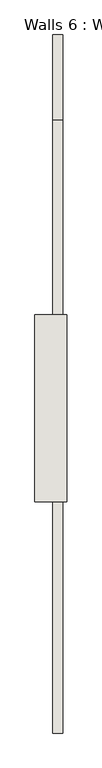
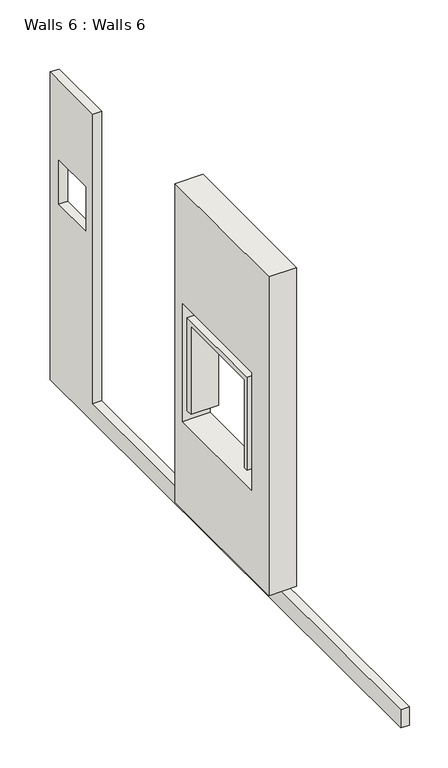
"""IFC4 building model written with IfcOpenShell, lengths in millimetres: wall geometry, Walls 6 : Walls 6."""

from ifc_helpers import new_model, si_unit, frame, origin, place, context, project, spatial, polyline, outline, extrude, source, transform, mapped, element, save


def walls_6_walls_6_5288b44a(model_context):
    return source(origin(), model_context, "Body", "SweptSolid", [
        extrude(outline(polyline([(9926.1302469, 14935.2), (9926.1302469, 10668.0), (9011.7302469, 10668.0), (1960.0609482, 10668.0), (1960.0609482, 10922.0), (8960.9302469, 10922.0), (8960.9302469, 14935.2), (9926.1302469, 14935.2)]), holes=[polyline([(9732.4609482, 13828.4684583), (9122.8609482, 13828.4684583), (9122.8609482, 13218.8684583), (9732.4609482, 13218.8684583), (9732.4609482, 13828.4684583)])]), frame((1662.3254876, 0.0, 0.0), z_axis=(1.0, 0.0, 0.0), x_axis=(0.0, 1.0, 0.0)), (0.0, 0.0, 1.0), 114.5722711),
        extrude(outline(polyline([(4601.6609482, 10972.8), (4601.6609482, 15392.4), (6735.2609482, 15392.4), (6735.2609482, 10972.8), (4601.6609482, 10972.8)]), holes=[polyline([(6572.7173646, 13824.3970745), (4997.9173646, 13824.3970745), (4997.9173646, 12192.0), (6572.7173646, 12192.0), (6572.7173646, 13824.3970745)])]), frame((1459.1254876, 0.0, 0.0), z_axis=(1.0, 0.0, 0.0), x_axis=(0.0, 1.0, 0.0)), (0.0, 0.0, 1.0), 363.6000013),
        extrude(outline(polyline([(6461.450673, 13699.1372891), (6461.450673, 12410.0872891), (6378.900673, 12410.0872891), (6378.900673, 13629.2872891), (5159.700673, 13629.2872891), (5159.700673, 12410.0872891), (5102.550673, 12410.0872891), (5102.550673, 13699.1372891), (6461.450673, 13699.1372891)])), frame((1459.1254876, 0.0, 0.0), z_axis=(1.0, 0.0, 0.0), x_axis=(0.0, 1.0, 0.0)), (0.0, 0.0, 1.0), 363.6000013),
    ])


if __name__ == "__main__":
    model = new_model("IFC4")
    model_context = context("Model", 3, world=origin())
    ifc_project = project(units=[si_unit("LENGTHUNIT", "METRE", prefix="MILLI")], contexts=[model_context])
    site = spatial("IfcSite", under=ifc_project)
    building = spatial("IfcBuilding", under=site)
    placement = place(None, origin())
    walls_6_walls_6_shape = walls_6_walls_6_5288b44a(model_context)
    element("IfcWall", 1, ObjectType="Walls 6 : Walls 6", at=placement, inside=building, context=model_context, shape_type="MappedRepresentation", body=[
        mapped(walls_6_walls_6_shape, transform((0.0, 0.0, 0.0), x_axis=(1.0, 0.0, 0.0), y_axis=(0.0, 1.0, 0.0), z_axis=(0.0, 0.0, 1.0))),
    ])
    save(model, "model.ifc")

# Revit data of these elements
# Element 1 (IfcWall, "Walls 6 : Walls 6")
#   Materials on its faces: "Default Wall"
# Materials
#   "Default Wall": colour RGB 128 128 128, transparency 0
